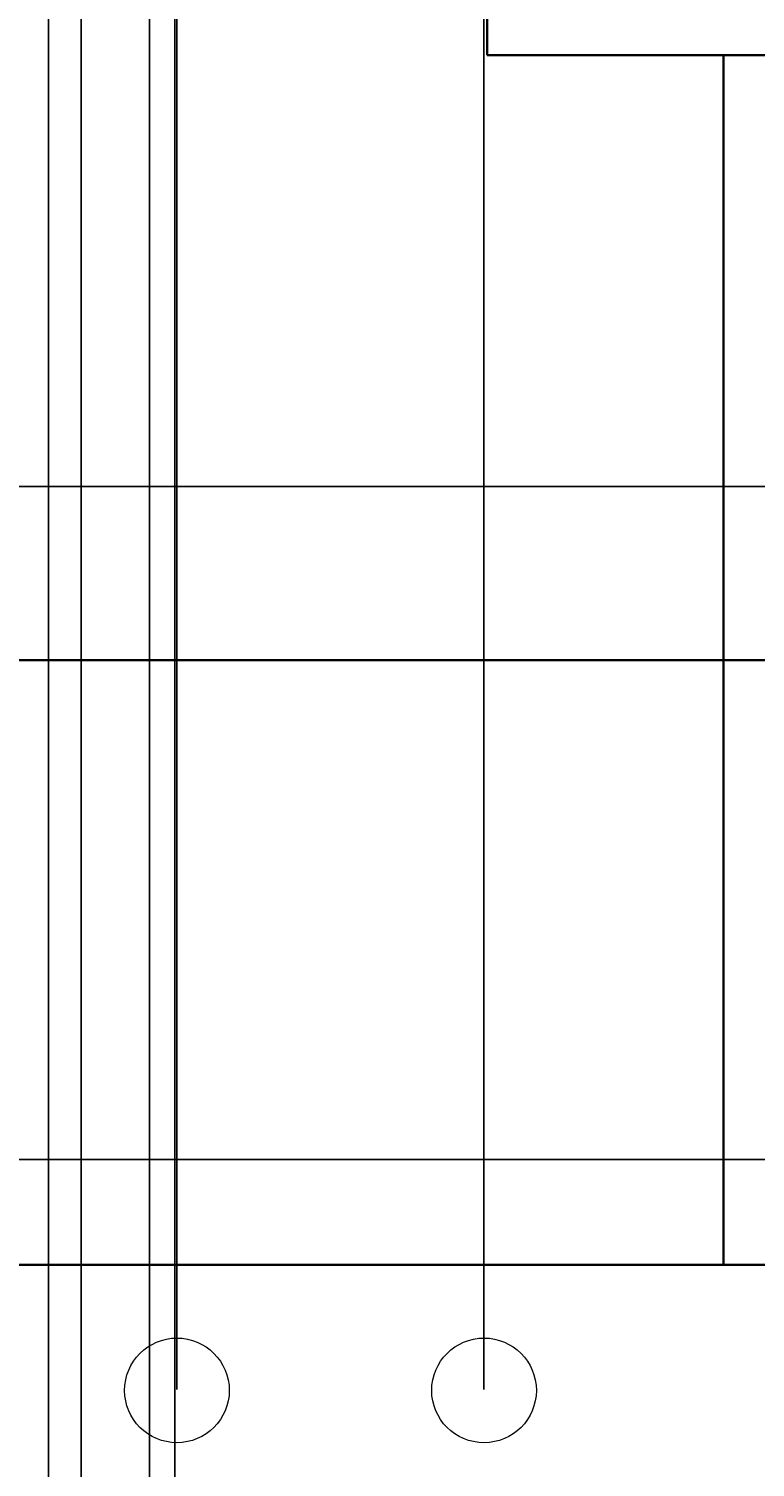
# Model space of a CAD drawing. Units: inches. Extents: x -13 to 809, y 112 to 656.
# Tile 33 of 55: x 257 to 314, y 446 to 561. Entities that reach past the tile are written whole.
import ezdxf

# ---------------------------------------------------------------- set-up
doc = ezdxf.new("R2010")
doc.units = ezdxf.units.IN
doc.header["$MEASUREMENT"] = 0
for name, color, linetype, lineweight in [('A-ANNO-DIMS', 2, 'Continuous', 18), ('A-ELEV', 7, 'Continuous', 35), ('A-ELEV-OTLN', 7, 'Continuous', 18)]:
    doc.layers.add(name, color=color, linetype=linetype, lineweight=lineweight)
doc.styles.get("Standard").update_dxf_attribs({"font": 'arial.ttf'})
doc.dimstyles.get("Standard").update_dxf_attribs({"dimtxt": 0.625, "dimasz": 0.18, "dimexe": 0.18, "dimexo": 0.0625, "dimgap": 0.09, "dimtad": 0, "dimtih": 1, "dimtoh": 1, "dimdec": 4, "dimzin": 0, "dimdsep": 46, "dimlunit": 4, "dimtxsty": 'Standard', "dimcen": 0.09, "dimadec": 0, "dimazin": 0, "dimtfac": 1, "dimtdec": 4, "dimtofl": 0, "dimtmove": 0, "dimatfit": 3, "dimfxl": 1, "dimtolj": 1, "dimtzin": 0, "dimarcsym": 0})

# ---------------------------------------------------------------- blocks, each defined once
blk = doc.blocks.new('*D23')
at = {"layer": 'A-ANNO-DIMS', "color": 0, "lineweight": -2, "transparency": 16777216}
for p, q in [((107.26, 510.58), (107.26, 655.96)), ((107.44, 655.78), (198.73, 655.78)), ((292.74, 655.78), (201.45, 655.78)), ((292.92, 569.3), (292.92, 655.96))]:
    blk.add_line(p, q, dxfattribs=at)
at = {"layer": 'A-ANNO-DIMS', "color": 0, "transparency": 16777216}
for points in [[(107.44, 655.81), (107.44, 655.75), (107.26, 655.78)], [(292.74, 655.81), (292.74, 655.75), (292.92, 655.78)]]:
    blk.add_solid(points, dxfattribs=at)
at = {"layer": 'Defpoints', "color": 0, "transparency": 16777216}
for p in [(292.92, 655.78), (292.92, 569.24), (107.26, 510.52)]:
    blk.add_point(p, dxfattribs=at)
at = {"layer": 'A-ANNO-DIMS', "color": 0, "transparency": 16777216, "insert": (200.09, 655.78), "char_height": 0.625, "attachment_point": 5}
blk.add_mtext('\\A1;185.66', dxfattribs=at)
blk = doc.blocks.new('*D25')
at = {"layer": 'A-ANNO-DIMS', "color": 0, "lineweight": -2, "transparency": 16777216}
for p, q in [((311.7, 617.43), (311.7, 655.96)), ((311.88, 655.78), (325.46, 655.78)), ((341.23, 655.78), (327.64, 655.78)), ((341.41, 524.34), (341.41, 655.96))]:
    blk.add_line(p, q, dxfattribs=at)
at = {"layer": 'A-ANNO-DIMS', "color": 0, "transparency": 16777216}
for points in [[(311.88, 655.81), (311.88, 655.75), (311.7, 655.78)], [(341.23, 655.81), (341.23, 655.75), (341.41, 655.78)]]:
    blk.add_solid(points, dxfattribs=at)
at = {"layer": 'Defpoints', "color": 0, "transparency": 16777216}
for p in [(341.41, 655.78), (311.7, 617.37), (341.41, 524.28)]:
    blk.add_point(p, dxfattribs=at)
at = {"layer": 'A-ANNO-DIMS', "color": 0, "transparency": 16777216, "insert": (326.55, 655.78), "char_height": 0.625, "attachment_point": 5}
blk.add_mtext('\\A1;29.71', dxfattribs=at)
blk = doc.blocks.new('*D36')
at = {"layer": 'A-ANNO-DIMS', "color": 0, "lineweight": -2, "transparency": 16777216}
for p, q in [((311.64, 569.24), (-12.1, 569.24)), ((-11.92, 569.06), (-11.92, 540.29)), ((-11.92, 510.7), (-11.92, 539.47)), ((107.2, 510.52), (-12.1, 510.52))]:
    blk.add_line(p, q, dxfattribs=at)
at = {"layer": 'A-ANNO-DIMS', "color": 0, "transparency": 16777216}
for points in [[(-11.95, 569.06), (-11.89, 569.06), (-11.92, 569.24)], [(-11.95, 510.7), (-11.89, 510.7), (-11.92, 510.52)]]:
    blk.add_solid(points, dxfattribs=at)
at = {"layer": 'Defpoints', "color": 0, "transparency": 16777216}
for p in [(-11.92, 569.24), (311.7, 569.24), (107.26, 510.52)]:
    blk.add_point(p, dxfattribs=at)
at = {"layer": 'A-ANNO-DIMS', "color": 0, "transparency": 16777216, "insert": (-11.92, 539.88), "char_height": 0.625, "attachment_point": 5}
blk.add_mtext('\\A1;58.72', dxfattribs=at)
blk = doc.blocks.new('*D39')
at = {"layer": 'A-ANNO-DIMS', "color": 0, "lineweight": -2, "transparency": 16777216}
for p, q in [((341.34, 524.28), (-12.1, 524.28)), ((-11.92, 524.1), (-11.92, 406.78)), ((-11.92, 288.63), (-11.92, 405.96)), ((341.34, 288.45), (-12.1, 288.45))]:
    blk.add_line(p, q, dxfattribs=at)
at = {"layer": 'A-ANNO-DIMS', "color": 0, "transparency": 16777216}
for points in [[(-11.95, 524.1), (-11.89, 524.1), (-11.92, 524.28)], [(-11.95, 288.63), (-11.89, 288.63), (-11.92, 288.45)]]:
    blk.add_solid(points, dxfattribs=at)
at = {"layer": 'Defpoints', "color": 0, "transparency": 16777216}
for p in [(-11.92, 524.28), (341.41, 524.28), (341.41, 288.45)]:
    blk.add_point(p, dxfattribs=at)
at = {"layer": 'A-ANNO-DIMS', "color": 0, "transparency": 16777216, "insert": (-11.92, 406.37), "char_height": 0.625, "attachment_point": 5}
blk.add_mtext('\\A1;235.83', dxfattribs=at)
blk = doc.blocks.new('*D43')
at = {"layer": 'A-ANNO-DIMS', "color": 0, "lineweight": -2, "transparency": 16777216}
for p, q in [((471.04, 470.88), (-12.1, 470.88)), ((-11.92, 470.7), (-11.92, 443.28)), ((-11.92, 415.04), (-11.92, 442.46)), ((471.04, 414.86), (-12.1, 414.86))]:
    blk.add_line(p, q, dxfattribs=at)
at = {"layer": 'A-ANNO-DIMS', "color": 0, "transparency": 16777216}
for points in [[(-11.95, 470.7), (-11.89, 470.7), (-11.92, 470.88)], [(-11.95, 415.04), (-11.89, 415.04), (-11.92, 414.86)]]:
    blk.add_solid(points, dxfattribs=at)
at = {"layer": 'Defpoints', "color": 0, "transparency": 16777216}
for p in [(-11.92, 470.88), (471.1, 470.88), (471.1, 414.86)]:
    blk.add_point(p, dxfattribs=at)
at = {"layer": 'A-ANNO-DIMS', "color": 0, "transparency": 16777216, "insert": (-11.92, 442.87), "char_height": 0.625, "attachment_point": 5}
blk.add_mtext('\\A1;56.02', dxfattribs=at)
blk = doc.blocks.new('*D100')
at = {"layer": 'A-ANNO-DIMS', "color": 0, "lineweight": -2, "transparency": 16777216}
for p, q in [((239.31, 452.63), (239.31, 655.96)), ((239.49, 655.78), (252.41, 655.78)), ((268.12, 655.78), (255.2, 655.78)), ((268.3, 452.63), (268.3, 655.96))]:
    blk.add_line(p, q, dxfattribs=at)
at = {"layer": 'A-ANNO-DIMS', "color": 0, "transparency": 16777216}
for points in [[(239.49, 655.81), (239.49, 655.75), (239.31, 655.78)], [(268.12, 655.81), (268.12, 655.75), (268.3, 655.78)]]:
    blk.add_solid(points, dxfattribs=at)
at = {"layer": 'Defpoints', "color": 0, "transparency": 16777216}
for p in [(268.3, 655.78), (239.31, 452.56), (268.3, 452.56)]:
    blk.add_point(p, dxfattribs=at)
at = {"layer": 'A-ANNO-DIMS', "color": 0, "transparency": 16777216, "insert": (253.8, 655.78), "char_height": 0.625, "attachment_point": 5}
blk.add_mtext('\\A1;28.994', dxfattribs=at)
blk = doc.blocks.new('*D101')
at = {"layer": 'A-ANNO-DIMS', "color": 0, "lineweight": -2, "transparency": 16777216}
for p, q in [((268.3, 452.63), (268.3, 655.96)), ((268.48, 655.78), (279.34, 655.78)), ((292.5, 655.78), (281.64, 655.78)), ((292.68, 452.63), (292.68, 655.96))]:
    blk.add_line(p, q, dxfattribs=at)
at = {"layer": 'A-ANNO-DIMS', "color": 0, "transparency": 16777216}
for points in [[(268.48, 655.81), (268.48, 655.75), (268.3, 655.78)], [(292.5, 655.81), (292.5, 655.75), (292.68, 655.78)]]:
    blk.add_solid(points, dxfattribs=at)
at = {"layer": 'Defpoints', "color": 0, "transparency": 16777216}
for p in [(292.68, 655.78), (268.3, 452.56), (292.68, 452.56)]:
    blk.add_point(p, dxfattribs=at)
at = {"layer": 'A-ANNO-DIMS', "color": 0, "transparency": 16777216, "insert": (280.49, 655.78), "char_height": 0.625, "attachment_point": 5}
blk.add_mtext('\\A1;24.38', dxfattribs=at)
blk = doc.blocks.new('*D102')
at = {"layer": 'A-ANNO-DIMS', "color": 0, "lineweight": -2, "transparency": 16777216}
for p, q in [((292.68, 452.63), (292.68, 655.96)), ((292.86, 655.78), (304.8, 655.78)), ((319.52, 655.78), (307.58, 655.78)), ((319.7, 452.63), (319.7, 655.96))]:
    blk.add_line(p, q, dxfattribs=at)
at = {"layer": 'A-ANNO-DIMS', "color": 0, "transparency": 16777216}
for points in [[(292.86, 655.81), (292.86, 655.75), (292.68, 655.78)], [(319.52, 655.81), (319.52, 655.75), (319.7, 655.78)]]:
    blk.add_solid(points, dxfattribs=at)
at = {"layer": 'Defpoints', "color": 0, "transparency": 16777216}
for p in [(319.7, 655.78), (292.68, 452.56), (319.7, 452.56)]:
    blk.add_point(p, dxfattribs=at)
at = {"layer": 'A-ANNO-DIMS', "color": 0, "transparency": 16777216, "insert": (306.19, 655.78), "char_height": 0.625, "attachment_point": 5}
blk.add_mtext('\\A1;27.017', dxfattribs=at)
blk = doc.blocks.new('*D116')
at = {"layer": 'A-ANNO-DIMS', "color": 0, "lineweight": -2, "transparency": 16777216}
for p, q in [((258.1, 210.85), (258.1, 655.96)), ((258.28, 655.78), (258.5, 655.78)), ((260.52, 655.78), (260.31, 655.78)), ((260.7, 207.43), (260.7, 655.96))]:
    blk.add_line(p, q, dxfattribs=at)
at = {"layer": 'A-ANNO-DIMS', "color": 0, "transparency": 16777216}
for points in [[(258.28, 655.81), (258.28, 655.75), (258.1, 655.78)], [(260.52, 655.81), (260.52, 655.75), (260.7, 655.78)]]:
    blk.add_solid(points, dxfattribs=at)
at = {"layer": 'Defpoints', "color": 0, "transparency": 16777216}
for p in [(260.7, 655.78), (258.1, 210.78), (260.7, 207.37)]:
    blk.add_point(p, dxfattribs=at)
at = {"layer": 'A-ANNO-DIMS', "color": 0, "transparency": 16777216, "insert": (259.4, 655.78), "char_height": 0.625, "attachment_point": 5}
blk.add_mtext('\\A1;2.60', dxfattribs=at)
blk = doc.blocks.new('*D119')
at = {"layer": 'A-ANNO-DIMS', "color": 0, "lineweight": -2, "transparency": 16777216}
for p, q in [((265.9486, 655.782835), (265.7686, 655.782835)), ((266.1286, 207.43492), (266.1286, 655.962835)), ((268.1286, 207.43492), (268.1286, 655.962835)), ((268.3086, 655.782835), (268.4886, 655.782835))]:
    blk.add_line(p, q, dxfattribs=at)
at = {"layer": 'A-ANNO-DIMS', "color": 0, "transparency": 16777216}
for points in [[(265.9486, 655.812835), (265.9486, 655.752835), (266.1286, 655.782835)], [(268.3086, 655.812835), (268.3086, 655.752835), (268.1286, 655.782835)]]:
    blk.add_solid(points, dxfattribs=at)
at = {"layer": 'Defpoints', "color": 0, "transparency": 16777216}
for p in [(268.1286, 655.782835), (266.1286, 207.37242), (268.1286, 207.37242)]:
    blk.add_point(p, dxfattribs=at)
at = {"layer": 'A-ANNO-DIMS', "color": 0, "transparency": 16777216, "insert": (267.1286, 655.782835), "char_height": 0.625, "attachment_point": 5}
blk.add_mtext('\\A1;2.00', dxfattribs=at)

msp = doc.modelspace()

# ---------------------------------------------------------------- linework, layer by layer
at = {"layer": 'A-ELEV'}
for p, q in [((292.923, 558.5199), (292.923, 569.2414)), ((341.4072, 558.5199), (292.923, 558.5199)), ((311.6991, 462.5199), (311.6991, 558.5199)), ((107.2588, 510.5199), (341.4072, 510.5199)), ((95.0469, 462.5199), (337.5074, 462.5199))]:
    msp.add_line(p, q, dxfattribs=at)
at = {"layer": 'A-ELEV-OTLN'}
for centre in [(268.3019, 452.5629), (292.6832, 452.5629)]:
    msp.add_circle(centre, 4.1542, dxfattribs=at)

# ---------------------------------------------------------------- dimensions: what is measured, and where the dimension line sits
at = {"layer": 'A-ANNO-DIMS'}
for base, p1, p2, override, picture, middle in [((292.923, 655.7828), (107.2588, 510.5199), (292.923, 569.2414), {"dimdec": 2, "dimlfac": 1, "dimrnd": 0, "dimzin": 0, "dimdsep": 46, "dimlunit": 2}, '*D23', (200.0909, 655.7828)), ((268.3019, 655.7828), (239.3079, 452.5629), (268.3019, 452.5629), {"dimdec": 3, "dimlfac": 1, "dimrnd": 0, "dimzin": 0, "dimdsep": 46, "dimlunit": 2}, '*D100', (253.8049, 655.7828)), ((260.7048, 655.7828), (258.1022, 210.7849), (260.7048, 207.3724), {"dimdec": 2, "dimlfac": 1, "dimrnd": 0, "dimzin": 0, "dimdsep": 46, "dimlunit": 2}, '*D116', (259.4035, 655.7828)), ((268.1286, 655.7828), (266.1286, 207.3724), (268.1286, 207.3724), {"dimdec": 2, "dimlfac": 1, "dimrnd": 0, "dimzin": 0, "dimdsep": 46, "dimlunit": 2}, '*D119', (267.1286, 655.7828)), ((292.6832, 655.7828), (268.3019, 452.5629), (292.6832, 452.5629), {"dimdec": 2, "dimlfac": 1, "dimrnd": 0, "dimzin": 0, "dimdsep": 46, "dimlunit": 2}, '*D101', (280.4925, 655.7828)), ((319.7004, 655.7828), (292.6832, 452.5629), (319.7004, 452.5629), {"dimdec": 3, "dimlfac": 1, "dimrnd": 0, "dimzin": 0, "dimdsep": 46, "dimlunit": 2}, '*D102', (306.1918, 655.7828)), ((341.4072, 655.7828), (311.6991, 617.3708), (341.4072, 524.281), {"dimdec": 2, "dimlfac": 1, "dimrnd": 0, "dimzin": 0, "dimdsep": 46, "dimlunit": 2}, '*D25', (326.5531, 655.7828))]:
    dim = msp.add_linear_dim(base=base, p1=p1, p2=p2, dimstyle='Standard', override=override, dxfattribs=at)
    dim.commit()
    dim.dimension.update_dxf_attribs({"geometry": picture, "text_midpoint": middle})
for base, p1, p2, picture, middle in [((-11.9191, 569.2414), (107.2588, 510.5199), (311.6991, 569.2414), '*D36', (-11.9191, 539.8806)), ((-11.9191, 524.281), (341.4072, 288.4508), (341.4072, 524.281), '*D39', (-11.9191, 406.3659)), ((-11.9191, 470.8765), (471.0998, 414.8594), (471.0998, 470.8765), '*D43', (-11.9191, 442.8679))]:
    dim = msp.add_linear_dim(base=base, p1=p1, p2=p2, angle=90, dimstyle='Standard', override={"dimdec": 2, "dimlfac": 1, "dimrnd": 0, "dimzin": 0, "dimdsep": 46, "dimlunit": 2}, dxfattribs=at)
    dim.commit()
    dim.dimension.update_dxf_attribs({"geometry": picture, "text_midpoint": middle})

doc.saveas('drawing.dxf')
